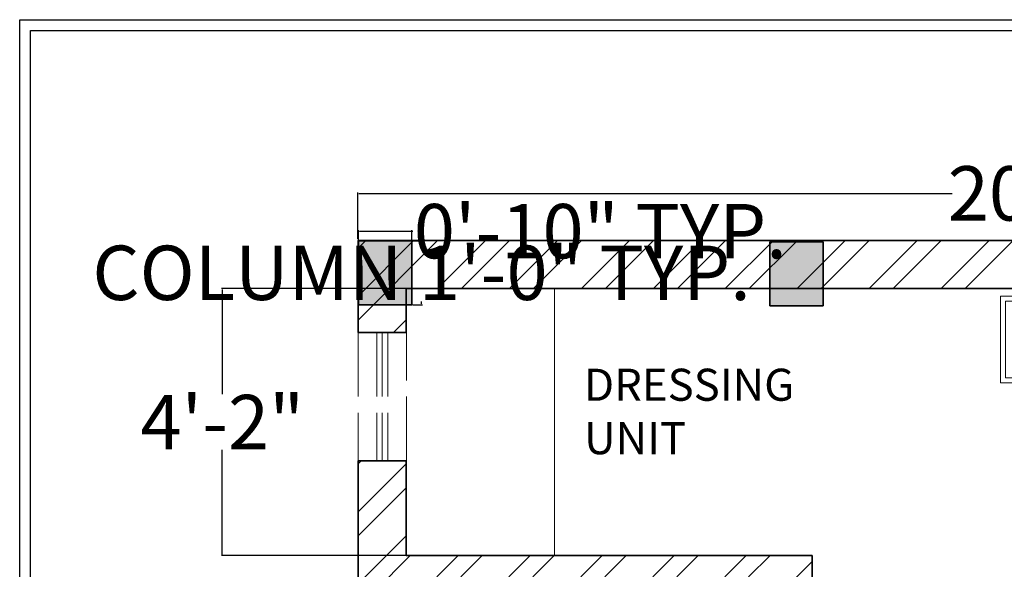
# Model space of a CAD drawing. Units: inches. Extents: x 1812 to 2791, y 2306 to 2959.
# Tile 7 of 8: x 2391 to 2575, y 2856 to 2959. Entities that reach past the tile are written whole.
import ezdxf

# ---------------------------------------------------------------- set-up
doc = ezdxf.new("R2010")
doc.units = ezdxf.units.IN
doc.linetypes.add('ACAD_ISO02W100', pattern=[15, 12, -3])
doc.layers.get('Defpoints').update_dxf_attribs({"lineweight": 50})
for name, color, linetype, lineweight in [('00 FURNITURE', 15, 'Continuous', 15), ('A-ANNO-DIMS', 2, 'Continuous', 18), ('A-ANNO-TTLB', 7, 'Continuous', 25), ('A-AREA-IDEN', 7, 'Continuous', 18), ('A-COLS', 7, 'Continuous', 35), ('A-FLOR-CASE', 8, 'Continuous', 18), ('A-GLAZ-VENT', 6, 'ACAD_ISO02W100', 13), ('A-WALL-PATT', 8, 'Continuous', 13), ('WALL', 7, 'Continuous', 35)]:
    doc.layers.add(name, color=color, linetype=linetype, lineweight=lineweight)
doc.styles.get("Standard").update_dxf_attribs({"font": 'arial.ttf'})
doc.dimstyles.get("Standard").update_dxf_attribs({"dimtxt": 10.18, "dimasz": 0.18, "dimexe": 0.18, "dimexo": 0.0625, "dimgap": 0.09, "dimtad": 0, "dimtih": 1, "dimtoh": 1, "dimdec": 0, "dimzin": 0, "dimdsep": 46, "dimlunit": 3, "dimtxsty": 'Standard', "dimcen": 0.09, "dimadec": 0, "dimazin": 0, "dimtfac": 1, "dimtdec": 0, "dimtofl": 0, "dimtmove": 0, "dimatfit": 3, "dimfxl": 1, "dimtolj": 1, "dimtzin": 0, "dimarcsym": 0})

# ---------------------------------------------------------------- blocks, each defined once
blk = doc.blocks.new('RGWTG')
at = {"layer": '00 FURNITURE'}
for p, q in [((578.36, 3473.58), (577.49, 3475.09)), ((578.23, 3473.51), (577.36, 3475.01)), ((578.23, 3473.58), (577.36, 3472.08)), ((578.36, 3473.51), (577.49, 3472)), ((578.29, 3473.62), (580.03, 3473.62)), ((578.29, 3473.47), (580.03, 3473.47)), ((521.93, 3464.58), (509.03, 3451.68)), ((509.93, 3464.58), (566.4, 3464.58)), ((557.53, 3463.84), (557.53, 3464.49)), ((557.53, 3464.49), (566.4, 3464.49)), ((558.2, 3464.49), (558.2, 3435.82)), ((559.57, 3464.49), (559.57, 3437.25)), ((560.94, 3464.49), (560.94, 3438.58)), ((562.3, 3464.49), (562.3, 3439.83)), ((563.67, 3464.49), (563.67, 3440.99)), ((565.04, 3464.49), (565.04, 3442.08)), ((566.4, 3464.58), (580.98, 3464.58)), ((566.4, 3464.49), (566.4, 3442.08)), ((566.4, 3464.49), (566.4, 3463.84)), ((580.98, 3464.58), (580.98, 3416.72)), ((509.03, 3422.63), (509.03, 3463.68)), ((558.2, 3426.48), (558.2, 3425.04)), ((509.03, 3400.68), (509.03, 3422.63)), ((558.2, 3416.13), (558.2, 3399.95)), ((580.98, 3416.72), (580.98, 3400.68)), ((559.57, 3414.75), (559.57, 3399.95)), ((560.94, 3413.39), (560.94, 3399.95)), ((562.3, 3412.04), (562.3, 3399.95)), ((563.67, 3410.72), (563.67, 3399.95)), ((580.08, 3399.78), (509.93, 3399.78)), ((557.53, 3399.95), (557.53, 3400.6)), ((566.4, 3399.95), (557.53, 3399.95)), ((566.4, 3400.6), (566.4, 3399.95)), ((578.23, 3390.78), (577.36, 3392.29)), ((578.36, 3390.86), (577.49, 3392.36)), ((578.23, 3390.86), (577.36, 3389.36)), ((578.36, 3390.78), (577.49, 3389.28)), ((578.29, 3390.9), (580.03, 3390.9)), ((578.29, 3390.74), (580.03, 3390.74))]:
    blk.add_line(p, q, dxfattribs=at)
for points in [[(568.43, 3465.48), (584.63, 3465.48), (584.63, 3481.68), (568.43, 3481.68)], [(569.33, 3466.38), (583.73, 3466.38), (583.73, 3480.78), (569.33, 3480.78)], [(580.98, 3399.78), (584.63, 3399.78), (584.63, 3464.58), (580.98, 3464.58)], [(568.43, 3398.88), (584.63, 3398.88), (584.63, 3382.68), (568.43, 3382.68)], [(569.33, 3397.98), (583.73, 3397.98), (583.73, 3383.58), (569.33, 3383.58)]]:
    blk.add_lwpolyline(points, close=True, dxfattribs=at)
for points in [[(566.52, 3464.49), (557.53, 3464.49), (557.53, 3435.08)], [(557.53, 3427.21), (557.53, 3424.3)], [(557.53, 3416.82), (557.53, 3399.95), (566.4, 3399.95), (566.4, 3409.94)]]:
    blk.add_lwpolyline(points, dxfattribs=at)
for centre, radius in [((578.29, 3473.54), 3.97), ((578.29, 3473.54), 3.63), ((578.29, 3473.54), 1.74), ((578.29, 3473.54), 1.56), ((578.29, 3390.82), 3.97), ((578.29, 3390.82), 3.63), ((578.29, 3390.82), 1.74), ((578.29, 3390.82), 1.56)]:
    blk.add_circle(centre, radius, dxfattribs=at)
for centre, radius, start, end in [((509.93, 3463.68), 0.9, 90, 180), ((529.65, 3456.88), 10.9, 135.0361, 191.9278), ((290.56, 3490.52), 268.3, 342.2214, 354.2925), ((516.73, 3443.97), 10.9, 78.0722, 134.9639), ((598.15, 3399.01), 54.32, 127.931, 142.069), ((566.05, 3440.57), 1.82, 45, 135), ((533.58, 3399.31), 54.32, 37.931, 52.069), ((574.84, 3431.77), 1.82, 315, 45), ((556.59, 3431.11), 1.82, 135, 225), ((598.15, 3388.23), 54.32, 127.931, 142.069), ((566.05, 3429.78), 1.82, 45, 135), ((533.58, 3388.53), 54.32, 37.931, 52.069), ((597.87, 3463.6), 54.32, 217.931, 224.141), ((533.28, 3463.88), 54.32, 316.32, 322.069), ((556.59, 3420.33), 1.82, 135, 225), ((574.84, 3420.99), 1.82, 315, 45), ((765.33, 3619.75), 290.45, 223.6069, 226.2326), ((533.28, 3453.1), 54.32, 307.931, 322.069), ((565.44, 3411.05), 1.47, 225.9674, 326.8337), ((545.02, 3395.29), 13.35, 20.4224, 85.5825), ((509.93, 3400.68), 0.9, 180, 270), ((580.08, 3400.68), 0.9, 270, 0)]:
    blk.add_arc(centre, radius, start, end, dxfattribs=at)
blk = doc.blocks.new('*D24')
at = {"layer": 'A-ANNO-DIMS', "color": 0, "lineweight": -2, "transparency": 16777216}
for p, q in [((2454.17, 2917.9), (2454.17, 2926.6)), ((2454.35, 2926.42), (2565.41, 2926.42)), ((2694.11, 2926.42), (2583.04, 2926.42)), ((2694.29, 2917.9), (2694.29, 2926.6))]:
    blk.add_line(p, q, dxfattribs=at)
at = {"layer": 'A-ANNO-DIMS', "color": 0, "transparency": 16777216}
for points in [[(2454.35, 2926.45), (2454.35, 2926.39), (2454.17, 2926.42)], [(2694.11, 2926.45), (2694.11, 2926.39), (2694.29, 2926.42)]]:
    blk.add_solid(points, dxfattribs=at)
at = {"layer": 'Defpoints', "color": 0, "transparency": 16777216}
for p in [(2694.29, 2926.42), (2454.17, 2917.83), (2694.29, 2917.83)]:
    blk.add_point(p, dxfattribs=at)
at = {"layer": 'A-ANNO-DIMS', "color": 0, "transparency": 16777216, "insert": (2574.23, 2926.42), "char_height": 10.18, "attachment_point": 5}
blk.add_mtext("\\A1;20'", dxfattribs=at)
blk = doc.blocks.new('COL')
at = {"transparency": 33554687}
h = blk.add_hatch(color=256, dxfattribs=at)
h.dxf.hatch_style = 1
h.paths.add_polyline_path([(2424.4, 2829.24), (2424.4, 2839.24), (2412.4, 2839.24), (2412.4, 2829.24)])
for p, q in [((2412.4, 2839.24), (2424.4, 2839.24)), ((2412.4, 2839.24), (2412.4, 2829.24)), ((2424.4, 2839.24), (2424.4, 2829.24)), ((2412.4, 2829.24), (2424.4, 2829.24))]:
    blk.add_line(p, q)
blk = doc.blocks.new('VENT-24x9')
for p, q in [((3.5, 24), (3.5, 0)), ((4.5, 24), (4.5, 0)), ((5.5, 24), (5.5, 0))]:
    blk.add_line(p, q)
blk.add_lwpolyline([(0, 0), (9, 0), (9, 24), (0, 24)], close=True)
blk = doc.blocks.new('SHEET-FRAME-RESIDENCE')
blk.add_lwpolyline([(0, 632.8), (378.76, 632.8), (378.76, 0), (0, 0)], close=True)
blk.add_lwpolyline([(2, 71.32), (2, 630.8), (376.76, 630.8), (376.76, 71.32)])
blk = doc.blocks.new('*D36')
at = {"layer": 'A-ANNO-DIMS', "color": 0, "lineweight": -2, "transparency": 16777216}
for p, q in [((2464.35, 2917.55), (2466.26, 2917.55)), ((2466.08, 2917.37), (2466.08, 2916.91)), ((2464.35, 2905.55), (2466.26, 2905.55)), ((2466.08, 2905.73), (2466.08, 2906.2))]:
    blk.add_line(p, q, dxfattribs=at)
at = {"layer": 'A-ANNO-DIMS', "color": 0, "transparency": 16777216}
for points in [[(2466.05, 2917.37), (2466.11, 2917.37), (2466.08, 2917.55)], [(2466.05, 2905.73), (2466.11, 2905.73), (2466.08, 2905.55)]]:
    blk.add_solid(points, dxfattribs=at)
at = {"layer": 'Defpoints', "color": 0, "transparency": 16777216}
for p in [(2464.28, 2917.55), (2464.28, 2905.55), (2466.08, 2905.55)]:
    blk.add_point(p, dxfattribs=at)
at = {"layer": 'A-ANNO-DIMS', "color": 0, "transparency": 16777216, "insert": (2466.08, 2911.55), "char_height": 10.18, "attachment_point": 5}
blk.add_mtext('\\A1;COLUMN 1\'-0" TYP.', dxfattribs=at)
blk = doc.blocks.new('*D37')
at = {"layer": 'A-ANNO-DIMS', "color": 0, "lineweight": -2, "transparency": 16777216}
for p, q in [((2454.28, 2917.62), (2454.28, 2919.53)), ((2454.46, 2919.35), (2464.1, 2919.35)), ((2464.28, 2917.62), (2464.28, 2919.53)), ((2464.28, 2919.35), (2464.46, 2919.35))]:
    blk.add_line(p, q, dxfattribs=at)
at = {"layer": 'A-ANNO-DIMS', "color": 0, "transparency": 16777216}
for points in [[(2454.46, 2919.38), (2454.46, 2919.32), (2454.28, 2919.35)], [(2464.1, 2919.38), (2464.1, 2919.32), (2464.28, 2919.35)]]:
    blk.add_solid(points, dxfattribs=at)
at = {"layer": 'Defpoints', "color": 0, "transparency": 16777216}
for p in [(2464.28, 2919.35), (2454.28, 2917.55), (2464.28, 2917.55)]:
    blk.add_point(p, dxfattribs=at)
at = {"layer": 'A-ANNO-DIMS', "color": 0, "transparency": 16777216, "insert": (2499.54, 2919.35), "char_height": 10.18, "attachment_point": 5}
blk.add_mtext('\\A1;0\'-10" TYP.', dxfattribs=at)
blk = doc.blocks.new('*D74')
at = {"layer": 'A-ANNO-DIMS', "color": 0, "lineweight": -2, "transparency": 16777216}
for p, q in [((2490.9, 2908.61), (2428.59, 2908.61)), ((2428.77, 2908.43), (2428.77, 2888.81)), ((2428.77, 2858.79), (2428.77, 2878.41)), ((2490.9, 2858.61), (2428.59, 2858.61))]:
    blk.add_line(p, q, dxfattribs=at)
at = {"layer": 'A-ANNO-DIMS', "color": 0, "transparency": 16777216}
for points in [[(2428.74, 2908.43), (2428.8, 2908.43), (2428.77, 2908.61)], [(2428.74, 2858.79), (2428.8, 2858.79), (2428.77, 2858.61)]]:
    blk.add_solid(points, dxfattribs=at)
at = {"layer": 'Defpoints', "color": 0, "transparency": 16777216}
for p in [(2490.96, 2908.61), (2428.77, 2858.61), (2490.96, 2858.61)]:
    blk.add_point(p, dxfattribs=at)
at = {"layer": 'A-ANNO-DIMS', "color": 0, "transparency": 16777216, "insert": (2428.77, 2883.61), "char_height": 10.18, "attachment_point": 5}
blk.add_mtext('\\A1;4\'-2"', dxfattribs=at)

msp = doc.modelspace()

# ---------------------------------------------------------------- hatches: boundary and pattern name
at = {"layer": 'A-WALL-PATT'}
h = msp.add_hatch(dxfattribs=at)
h.set_pattern_fill('ANSI32', color=256)
h.set_pattern_definition([(45, (563.806, 20.011), (-6.735192, 6.735192), []), (45, (568.296, 20.011), (-6.735192, 6.735192), [])])
h.paths.add_polyline_path([(2694.19, 2437.61), (2683.5, 2437.61), (2683.5, 2788.57), (2685.19, 2788.57), (2685.19, 2821.64), (2685.13, 2869.37), (2685.13, 2821.64), (2694.19, 2821.64)])
h.paths.add_polyline_path([(2587.19, 2446.61), (2463.19, 2446.61), (2463.19, 2473.61), (2515.61, 2473.61), (2515.61, 2477.61), (2463.19, 2477.61), (2463.19, 2610.61), (2523.74, 2610.61), (2523.74, 2614.61), (2463.19, 2614.61), (2463.19, 2654.54), (2454.19, 2654.54), (2454.19, 2437.61), (2587.19, 2437.61)])
h.paths.add_polyline_path([(2683.5, 2446.61), (2676.19, 2446.61), (2676.19, 2437.61), (2683.5, 2437.61)])
h.paths.add_polyline_path([(2463.19, 2760.61), (2505.19, 2760.61), (2505.19, 2764.61), (2463.19, 2764.61), (2463.19, 2792.95), (2454.19, 2792.95), (2454.19, 2702.54), (2463.02, 2702.54), (2463.02, 2702.65)])
h.paths.add_polyline_path([(2539.19, 2858.61), (2463.19, 2858.61), (2463.19, 2876.35), (2454.19, 2876.35), (2454.19, 2816.96), (2463.19, 2816.96), (2463.19, 2854.61), (2535.19, 2854.61), (2535.19, 2760.61), (2539.19, 2760.61)])
h.paths.add_polyline_path([(2683.5, 2917.61), (2454.19, 2917.61), (2454.19, 2900.37), (2463.19, 2900.37), (2463.19, 2908.61), (2683.5, 2908.61)])
h.paths.add_polyline_path([(2694.19, 2917.61), (2683.5, 2917.61), (2683.5, 2908.61), (2685.19, 2908.61), (2685.19, 2869.64), (2694.19, 2869.64)])

# ---------------------------------------------------------------- linework, layer by layer
at = {"layer": 'A-FLOR-CASE'}
msp.add_line((2490.96, 2908.61), (2490.96, 2858.61), dxfattribs=at)
at = {"layer": 'WALL'}
for p, q in [((2454.19, 2917.61), (2694.19, 2917.61)), ((2454.19, 2900.35), (2454.19, 2917.61)), ((2463.19, 2908.61), (2685.19, 2908.61)), ((2463.19, 2900.35), (2463.19, 2908.61)), ((2454.19, 2900.35), (2463.19, 2900.35)), ((2454.19, 2816.95), (2454.19, 2876.35)), ((2454.19, 2876.35), (2463.19, 2876.35)), ((2463.19, 2858.61), (2463.19, 2876.35)), ((2463.19, 2858.61), (2539.19, 2858.61)), ((2539.19, 2760.61), (2539.19, 2858.61))]:
    msp.add_line(p, q, dxfattribs=at)

# ---------------------------------------------------------------- block references
at = {"layer": '00 FURNITURE', "xscale": -1, "rotation": 270}
msp.add_blockref('RGWTG', (-808.2, 2322.54), dxfattribs=at)
at = {"layer": 'A-ANNO-TTLB'}
msp.add_blockref('SHEET-FRAME-RESIDENCE', (2390.83, 2326.13), dxfattribs=at)
at = {"layer": 'A-COLS', "rotation": 270}
for p in [(-374.96, 5329.95), (-297.97, 5329.77)]:
    msp.add_blockref('COL', p, dxfattribs=at)
at = {"layer": 'A-GLAZ-VENT'}
msp.add_blockref('VENT-24x9', (2454.23, 2876.37), dxfattribs=at)

# ---------------------------------------------------------------- texts
at = {"layer": 'A-AREA-IDEN', "insert": (2496.5, 2893.6), "char_height": 6, "attachment_point": 1}
msp.add_mtext_dynamic_manual_height_columns('DRESSING\\PUNIT', width=184.4395, gutter_width=12.5, heights=[0], dxfattribs=at)

# ---------------------------------------------------------------- dimensions: what is measured, and where the dimension line sits
at = {"layer": 'A-ANNO-DIMS'}
dim = msp.add_linear_dim(base=(2466.08, 2905.55), p1=(2464.28, 2917.55), p2=(2464.28, 2905.55), angle=270, text='COLUMN <> TYP.', dimstyle='Standard', override={"dimdec": 1, "dimlfac": 1, "dimrnd": 0, "dimzin": 1, "dimdsep": 46, "dimlunit": 4, "dimfrac": 2}, dxfattribs=at)
dim.commit()
dim.dimension.update_dxf_attribs({"geometry": '*D36', "text_midpoint": (2466.08, 2911.55)})
dim = msp.add_linear_dim(base=(2694.29, 2926.42), p1=(2454.17, 2917.83), p2=(2694.29, 2917.83), dimstyle='Standard', override={"dimclrd": 0, "dimclre": 0, "dimclrt": 0}, dxfattribs=at)
dim.commit()
dim.dimension.update_dxf_attribs({"geometry": '*D24', "text_midpoint": (2574.23, 2926.42)})
dim = msp.add_linear_dim(base=(2464.28, 2919.35), p1=(2454.28, 2917.55), p2=(2464.28, 2917.55), text='<> TYP.', dimstyle='Standard', override={"dimdec": 1, "dimlfac": 1, "dimrnd": 0, "dimzin": 1, "dimdsep": 46, "dimlunit": 4, "dimfrac": 2}, dxfattribs=at)
dim.commit()
dim.dimension.update_dxf_attribs({"geometry": '*D37', "text_midpoint": (2499.54, 2919.35)})
dim = msp.add_linear_dim(base=(2428.77, 2858.61), p1=(2490.96, 2908.61), p2=(2490.96, 2858.61), angle=90, dimstyle='Standard', override={"dimdec": 1, "dimlfac": 1, "dimrnd": 0, "dimzin": 1, "dimdsep": 46, "dimlunit": 4, "dimfrac": 2}, dxfattribs=at)
dim.commit()
dim.dimension.update_dxf_attribs({"geometry": '*D74', "text_midpoint": (2428.77, 2883.61)})

doc.saveas('drawing.dxf')
